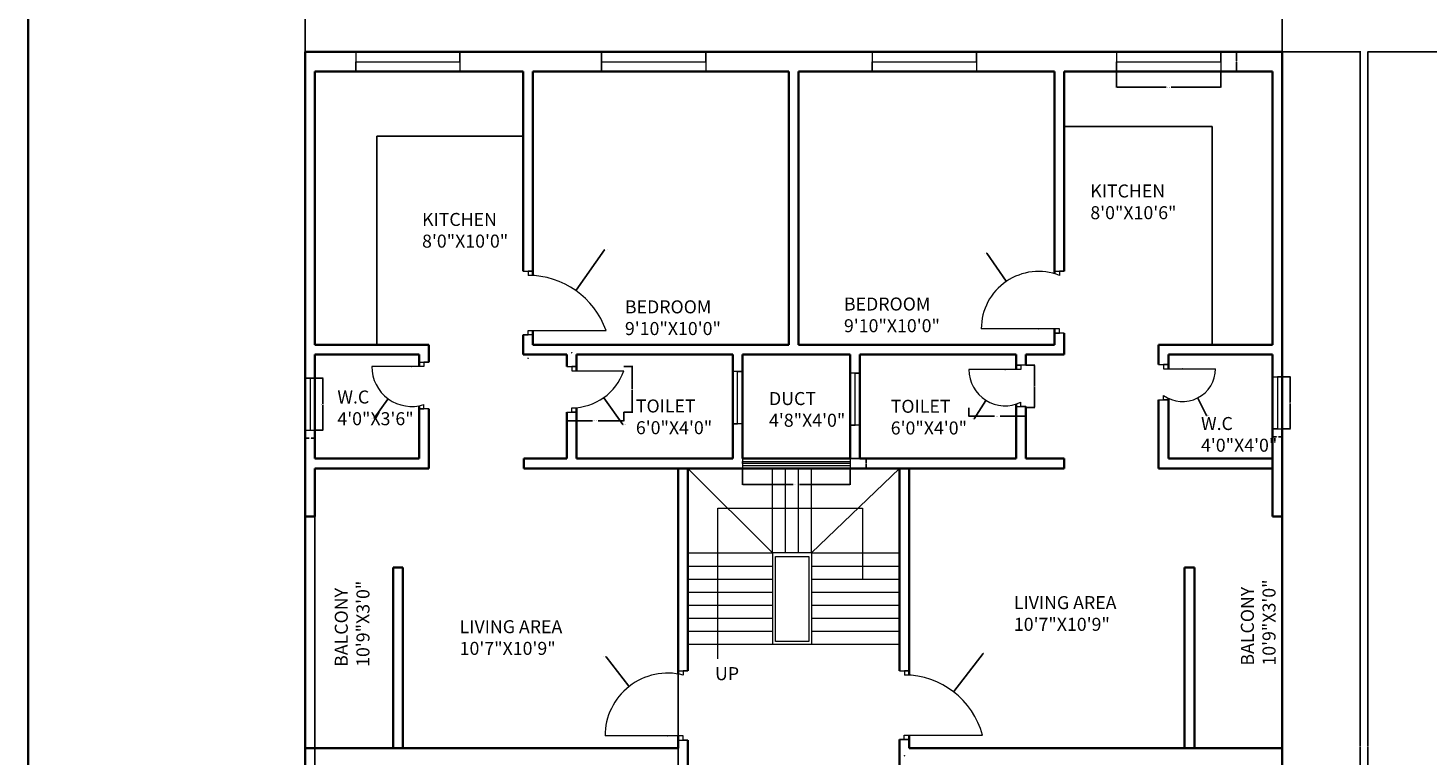
# Model space of a CAD drawing. Units: inches. Extents: x 2043 to 3387, y 1535 to 2797.
# Tile 2 of 7: x 2043 to 2688, y 2002 to 2337. Entities that reach past the tile are written whole.
import ezdxf

# ---------------------------------------------------------------- set-up
doc = ezdxf.new("R2010")
doc.units = ezdxf.units.IN
for name, color, linetype, lineweight in [('A-ANNO-DIMS', 2, 'Continuous', 18), ('A-ANNO-TEXT', 7, 'Continuous', 18), ('A-ANNO-TTLB', 7, 'Continuous', 35), ('A-AREA-IDEN', 7, 'Continuous', 18), ('A-DOOR', 3, 'Continuous', 18), ('A-FLOR-FIXT', 9, 'Continuous', 25), ('A-FLOR-STRS', 2, 'Continuous', 18), ('A-GLAZ', 4, 'Continuous', 18), ('A-WALL', 7, 'Continuous', 35)]:
    doc.layers.add(name, color=color, linetype=linetype, lineweight=lineweight)
doc.styles.get("Standard").update_dxf_attribs({"font": 'arial.ttf'})
doc.dimstyles.get("Standard").update_dxf_attribs({"dimtxt": 0.18, "dimasz": 0.18, "dimexe": 0.18, "dimexo": 0.0625, "dimgap": 0.09, "dimtad": 0, "dimtih": 1, "dimtoh": 1, "dimdec": 4, "dimzin": 0, "dimdsep": 46, "dimtxsty": 'Standard', "dimcen": 0.09, "dimadec": 0, "dimazin": 0, "dimtfac": 1, "dimtdec": 4, "dimtofl": 0, "dimtmove": 0, "dimatfit": 3, "dimfxl": 1, "dimtolj": 1, "dimtzin": 0, "dimarcsym": 0})

# ---------------------------------------------------------------- blocks, each defined once
blk = doc.blocks.new('DOOR-24-WC-NW')
for p, q in [((24, 19.53), (0, 19.53)), ((21.75, 21.53), (26.25, 21.53)), ((26.25, 21.53), (24, 21.53)), ((24, 21.53), (24, 19.53)), ((24, 0), (24, 2)), ((26.25, 0), (21.75, 0)), ((21.75, 0), (24, 0))]:
    blk.add_line(p, q)
blk.add_arc((18.4, 19.53), 18.41, 180, 287.6967)
blk = doc.blocks.new('DOOR-36-BED-NW')
for p, q in [((0, 29.41), (4.5, 29.41)), ((4.5, 29.41), (2.25, 29.41)), ((2.25, 29.41), (2.25, 27.41)), ((4.5, 0), (0, 0)), ((0, 0), (2.25, 0)), ((2.25, 0), (2.25, 2)), ((2.25, 2), (38.25, 2))]:
    blk.add_line(p, q)
blk.add_arc((2.25, -10.79), 38.2, 19.56074, 90)
blk = doc.blocks.new('DOOR-36-BED-NE')
for p, q in [((33.75, 28.58), (38.25, 28.58)), ((38.25, 28.58), (36, 28.58)), ((36, 28.58), (36, 26.58)), ((36, 2), (0, 2)), ((38.25, 0), (33.75, 0)), ((33.75, 0), (36, 0)), ((36, 0), (36, 2))]:
    blk.add_line(p, q)
blk.add_arc((26.39, 2), 26.39, 68.64806, 180)
blk = doc.blocks.new('DOOR-24-WC-NE')
for p, q in [((0, 17.14), (4.5, 17.14)), ((4.5, 17.14), (2.25, 17.14)), ((2.25, 17.14), (2.25, 15.14)), ((2.25, 15.14), (26.25, 15.14)), ((0, 0.86), (4.5, 0.86)), ((2.25, 0.86), (2.25, 2.86)), ((4.5, 0.86), (2.25, 0.86)), ((4.5, 0.86), (4.5, 0.86))]:
    blk.add_line(p, q)
blk.add_arc((11.11, 15.14), 15.14, 234.19542, 0)
blk = doc.blocks.new('DOOR-24-BATH-NW')
for p, q in [((0, 21.1), (4.5, 21.1)), ((4.5, 21.1), (2.25, 21.1)), ((2.25, 21.1), (2.25, 19.1)), ((2.25, 19.1), (26.25, 19.1)), ((2.25, 0), (2.25, 2)), ((0, 0), (4.5, 0)), ((4.5, 0), (2.25, 0))]:
    blk.add_line(p, q)
blk.add_arc((2.25, 27.39), 25.39, 270, 340.93831)
blk = doc.blocks.new('DOOR-24-BATH-NE')
for p, q in [((24, 17.07), (0, 17.07)), ((26.25, 19.07), (21.75, 19.07)), ((21.75, 19.07), (24, 19.07)), ((24, 19.07), (24, 17.07)), ((24, 0), (24, 2)), ((21.75, 0), (26.25, 0)), ((26.25, 0), (24, 0))]:
    blk.add_line(p, q)
blk.add_arc((16.73, 17.07), 16.73, 180, 295.74666)
blk = doc.blocks.new('DOOR-36-ENTRY-NW')
for p, q in [((33.75, 32.08), (38.25, 32.08)), ((38.25, 32.08), (36, 32.08)), ((36, 32.08), (36, 30.08)), ((36, 2), (0, 2)), ((33.75, 0), (38.25, 0)), ((36, 0), (36, 2)), ((38.25, 0), (36, 0))]:
    blk.add_line(p, q)
blk.add_arc((28.95, 2), 28.95, 75.89964, 180)
blk = doc.blocks.new('DOOR-36-ENTRY-NE')
for p, q in [((0, 31.7), (3.27, 31.7)), ((4.5, 31.7), (2.28, 31.7)), ((2.28, 31.7), (2.28, 29.7)), ((3.27, 31.7), (4.5, 31.7)), ((0, 0), (4.5, 0)), ((4.5, 0), (0, 0)), ((0, 0), (2.25, 0)), ((2.25, 0), (2.25, 2)), ((2.25, 2), (38.25, 2))]:
    blk.add_line(p, q)
blk.add_arc((2.28, -7.5), 37.2, 14.79344, 90)
blk = doc.blocks.new('COUNTER-L-NW')
for p, q in [((67.52, 96.23), (0, 96.23)), ((0, 96.23), (0, 0))]:
    blk.add_line(p, q)
blk = doc.blocks.new('COUNTER-L-NE')
for p, q in [((0, 100.61), (68.19, 100.61)), ((68.19, 100.61), (68.19, 0))]:
    blk.add_line(p, q)
blk = doc.blocks.new('STAIR-U-RETURN')
for p, q in [((0, 87.81), (0, 48.81)), ((39, 48.81), (0, 87.81)), ((39, 48.81), (39, 87.81)), ((45, 48.81), (45, 87.81)), ((51, 48.81), (51, 87.81)), ((57, 48.81), (57, 87.81)), ((57, 48.81), (97.5, 87.81)), ((97.5, 87.81), (58.5, 87.81)), ((13.82, 0), (13.82, 69.54)), ((13.82, 69.54), (80.42, 69.54)), ((80.42, 69.54), (80.42, 36.81)), ((0, 48.81), (39, 48.81)), ((57, 48.81), (39, 48.81)), ((39, 48.81), (39, 48.81)), ((39, 48.81), (39, 6.81)), ((57, 48.81), (57, 6.81)), ((57, 48.81), (97.5, 48.81)), ((0, 42.81), (39, 42.81)), ((57, 42.81), (97.5, 42.81)), ((0, 36.81), (39, 36.81)), ((57, 36.81), (97.5, 36.81)), ((0, 30.81), (39, 30.81)), ((57, 30.81), (97.5, 30.81)), ((0, 24.81), (39, 24.81)), ((57, 24.81), (97.5, 24.81)), ((0, 18.81), (39, 18.81)), ((57, 18.81), (97.5, 18.81)), ((0, 12.81), (39, 12.81)), ((0, 6.81), (39, 6.81)), ((39, 6.81), (57, 6.81)), ((57, 12.81), (97.5, 12.81)), ((57, 6.81), (97.5, 6.81))]:
    blk.add_line(p, q)
blk.add_lwpolyline([(40.29, 47.17), (55.75, 47.17), (55.75, 8.03), (40.29, 8.03)], close=True)
blk = doc.blocks.new('WIN-48-PLAN')
for p, q in [((0, 9), (0, 0)), ((48, 4.5), (48, 9)), ((48, 9), (48, 0)), ((0, 0), (0, 4.5)), ((0, 4.5), (48, 4.5))]:
    blk.add_line(p, q)
blk = doc.blocks.new('WIN-48-N-JAMB')
for p, q in [((0, 9), (0, 0)), ((0, 0), (0, 9)), ((0, 9), (0, 4.5)), ((48, 4.5), (48, 9)), ((48, 9), (48, 0)), ((0, 4.5), (48, 4.5))]:
    blk.add_line(p, q)
blk = doc.blocks.new('VENT-24-W')
for p, q in [((0, 24), (4.5, 24)), ((4.5, 24), (0, 24)), ((0, 24), (0, 0)), ((2.25, 24), (2.25, 0)), ((0, 0), (4.5, 0))]:
    blk.add_line(p, q)
blk = doc.blocks.new('VENT-24-PLAN')
for p, q in [((0, 24), (4.5, 24)), ((4.5, 24), (2.25, 24)), ((2.25, 24), (2.25, 0)), ((2.25, 0), (0, 0)), ((0, 0), (4.5, 0))]:
    blk.add_line(p, q)
blk = doc.blocks.new('WIN-STAIR-DUCT')
for p, q in [((0, 4.5), (0, 0)), ((0, 2.25), (0, 3.25)), ((0, 3.25), (49.62, 3.25)), ((49.62, 2.25), (0, 2.25)), ((49.62, 1.25), (0, 1.25)), ((49.62, 4.5), (49.62, 0)), ((49.62, 3.25), (49.62, 2.25)), ((49.62, 2.25), (49.62, 2.25)), ((49.62, 2.25), (49.62, 1.25))]:
    blk.add_line(p, q)
blk = doc.blocks.new('*D35')
at = {"layer": 'A-ANNO-DIMS', "color": 0, "lineweight": -2, "transparency": 16777216}
for p, q in [((2620.91, 2176.55), (2624.63, 2176.55)), ((2624.45, 2176.37), (2624.45, 2164.73)), ((2624.45, 2152.73), (2624.45, 2164.37)), ((2620.91, 2152.55), (2624.63, 2152.55))]:
    blk.add_line(p, q, dxfattribs=at)
at = {"layer": 'A-ANNO-DIMS', "color": 0, "transparency": 16777216}
for points in [[(2624.42, 2176.37), (2624.48, 2176.37), (2624.45, 2176.55)], [(2624.42, 2152.73), (2624.48, 2152.73), (2624.45, 2152.55)]]:
    blk.add_solid(points, dxfattribs=at)
at = {"layer": 'Defpoints', "color": 0, "transparency": 16777216}
for p in [(2620.85, 2176.55), (2624.45, 2176.55), (2620.85, 2152.55)]:
    blk.add_point(p, dxfattribs=at)
at = {"layer": 'A-ANNO-DIMS', "color": 0, "transparency": 16777216, "insert": (2624.45, 2164.55), "char_height": 0.18, "attachment_point": 5}
blk.add_mtext('\\A1;VENT 24 TYP.', dxfattribs=at)
blk = doc.blocks.new('*D36')
at = {"layer": 'A-ANNO-DIMS', "color": 0, "lineweight": -2, "transparency": 16777216}
for p, q in [((2616.35, 2152.48), (2616.35, 2148.77)), ((2620.85, 2152.48), (2620.85, 2148.77)), ((2616.53, 2148.95), (2618.14, 2148.95)), ((2620.67, 2148.95), (2619.06, 2148.95))]:
    blk.add_line(p, q, dxfattribs=at)
at = {"layer": 'A-ANNO-DIMS', "color": 0, "transparency": 16777216}
for points in [[(2616.53, 2148.98), (2616.53, 2148.92), (2616.35, 2148.95)], [(2620.67, 2148.98), (2620.67, 2148.92), (2620.85, 2148.95)]]:
    blk.add_solid(points, dxfattribs=at)
at = {"layer": 'Defpoints', "color": 0, "transparency": 16777216}
for p in [(2616.35, 2152.55), (2620.85, 2152.55), (2620.85, 2148.95)]:
    blk.add_point(p, dxfattribs=at)
at = {"layer": 'A-ANNO-DIMS', "color": 0, "transparency": 16777216, "insert": (2618.6, 2148.95), "char_height": 0.18, "attachment_point": 5}
blk.add_mtext('\\A1;5 TYP.', dxfattribs=at)
blk = doc.blocks.new('*D37')
at = {"layer": 'A-ANNO-DIMS', "color": 0, "lineweight": -2, "transparency": 16777216}
for p, q in [((2544.5, 2317.31), (2544.5, 2310)), ((2592.5, 2317.31), (2592.5, 2310)), ((2544.68, 2310.18), (2567.38, 2310.18)), ((2592.32, 2310.18), (2569.62, 2310.18))]:
    blk.add_line(p, q, dxfattribs=at)
at = {"layer": 'A-ANNO-DIMS', "color": 0, "transparency": 16777216}
for points in [[(2544.68, 2310.21), (2544.68, 2310.15), (2544.5, 2310.18)], [(2592.32, 2310.21), (2592.32, 2310.15), (2592.5, 2310.18)]]:
    blk.add_solid(points, dxfattribs=at)
at = {"layer": 'Defpoints', "color": 0, "transparency": 16777216}
for p in [(2544.5, 2317.38), (2592.5, 2317.38), (2592.5, 2310.18)]:
    blk.add_point(p, dxfattribs=at)
at = {"layer": 'A-ANNO-DIMS', "color": 0, "transparency": 16777216, "insert": (2568.5, 2310.18), "char_height": 0.18, "attachment_point": 5}
blk.add_mtext('\\A1;WINDOW 48 TYP.', dxfattribs=at)
blk = doc.blocks.new('*D38')
at = {"layer": 'A-ANNO-DIMS', "color": 0, "lineweight": -2, "transparency": 16777216}
for p, q in [((2592.57, 2326.38), (2599.88, 2326.38)), ((2599.7, 2326.2), (2599.7, 2322.06)), ((2599.7, 2317.56), (2599.7, 2321.7)), ((2592.57, 2317.38), (2599.88, 2317.38))]:
    blk.add_line(p, q, dxfattribs=at)
at = {"layer": 'A-ANNO-DIMS', "color": 0, "transparency": 16777216}
for points in [[(2599.67, 2326.2), (2599.73, 2326.2), (2599.7, 2326.38)], [(2599.67, 2317.56), (2599.73, 2317.56), (2599.7, 2317.38)]]:
    blk.add_solid(points, dxfattribs=at)
at = {"layer": 'Defpoints', "color": 0, "transparency": 16777216}
for p in [(2592.5, 2326.38), (2599.7, 2326.38), (2592.5, 2317.38)]:
    blk.add_point(p, dxfattribs=at)
at = {"layer": 'A-ANNO-DIMS', "color": 0, "transparency": 16777216, "insert": (2599.7, 2321.88), "char_height": 0.18, "attachment_point": 5}
blk.add_mtext('\\A1;9 TYP.', dxfattribs=at)
blk = doc.blocks.new('*D43')
at = {"layer": 'A-ANNO-DIMS', "color": 0, "lineweight": -2, "transparency": 16777216}
for p, q in [((2174.91, 2175.93), (2178.63, 2175.93)), ((2178.45, 2175.75), (2178.45, 2164.11)), ((2178.45, 2152.11), (2178.45, 2163.75)), ((2174.91, 2151.93), (2178.63, 2151.93))]:
    blk.add_line(p, q, dxfattribs=at)
at = {"layer": 'A-ANNO-DIMS', "color": 0, "transparency": 16777216}
for points in [[(2178.42, 2175.75), (2178.48, 2175.75), (2178.45, 2175.93)], [(2178.42, 2152.11), (2178.48, 2152.11), (2178.45, 2151.93)]]:
    blk.add_solid(points, dxfattribs=at)
at = {"layer": 'Defpoints', "color": 0, "transparency": 16777216}
for p in [(2174.85, 2175.93), (2178.45, 2175.93), (2174.85, 2151.93)]:
    blk.add_point(p, dxfattribs=at)
at = {"layer": 'A-ANNO-DIMS', "color": 0, "transparency": 16777216, "insert": (2178.45, 2163.93), "char_height": 0.18, "attachment_point": 5}
blk.add_mtext('\\A1;VENT 24 TYP.', dxfattribs=at)
blk = doc.blocks.new('*D44')
at = {"layer": 'A-ANNO-DIMS', "color": 0, "lineweight": -2, "transparency": 16777216}
for p, q in [((2170.35, 2151.87), (2170.35, 2148.15)), ((2174.85, 2151.87), (2174.85, 2148.15)), ((2170.53, 2148.33), (2172.14, 2148.33)), ((2174.67, 2148.33), (2173.06, 2148.33))]:
    blk.add_line(p, q, dxfattribs=at)
at = {"layer": 'A-ANNO-DIMS', "color": 0, "transparency": 16777216}
for points in [[(2170.53, 2148.36), (2170.53, 2148.3), (2170.35, 2148.33)], [(2174.67, 2148.36), (2174.67, 2148.3), (2174.85, 2148.33)]]:
    blk.add_solid(points, dxfattribs=at)
at = {"layer": 'Defpoints', "color": 0, "transparency": 16777216}
for p in [(2170.35, 2151.93), (2174.85, 2151.93), (2174.85, 2148.33)]:
    blk.add_point(p, dxfattribs=at)
at = {"layer": 'A-ANNO-DIMS', "color": 0, "transparency": 16777216, "insert": (2172.6, 2148.33), "char_height": 0.18, "attachment_point": 5}
blk.add_mtext('\\A1;5 TYP.', dxfattribs=at)
blk = doc.blocks.new('*D45')
at = {"layer": 'A-ANNO-DIMS', "color": 0, "lineweight": -2, "transparency": 16777216}
for p, q in [((2372.01, 2134.31), (2372.01, 2126.75)), ((2421.63, 2134.31), (2421.63, 2126.75)), ((2372.19, 2126.93), (2395.32, 2126.93)), ((2421.45, 2126.93), (2398.31, 2126.93))]:
    blk.add_line(p, q, dxfattribs=at)
at = {"layer": 'A-ANNO-DIMS', "color": 0, "transparency": 16777216}
for points in [[(2372.19, 2126.96), (2372.19, 2126.9), (2372.01, 2126.93)], [(2421.45, 2126.96), (2421.45, 2126.9), (2421.63, 2126.93)]]:
    blk.add_solid(points, dxfattribs=at)
at = {"layer": 'Defpoints', "color": 0, "transparency": 16777216}
for p in [(2372.01, 2134.38), (2421.63, 2134.38), (2421.63, 2126.93)]:
    blk.add_point(p, dxfattribs=at)
at = {"layer": 'A-ANNO-DIMS', "color": 0, "transparency": 16777216, "insert": (2396.82, 2126.93), "char_height": 0.18, "attachment_point": 5}
blk.add_mtext('\\A1;DUCT WINDOW 50 TYP.', dxfattribs=at)
blk = doc.blocks.new('*D46')
at = {"layer": 'A-ANNO-DIMS', "color": 0, "lineweight": -2, "transparency": 16777216}
for p, q in [((2421.69, 2138.88), (2429.25, 2138.88)), ((2429.07, 2138.7), (2429.07, 2136.81)), ((2421.69, 2134.38), (2429.25, 2134.38)), ((2429.07, 2134.56), (2429.07, 2136.45))]:
    blk.add_line(p, q, dxfattribs=at)
at = {"layer": 'A-ANNO-DIMS', "color": 0, "transparency": 16777216}
for points in [[(2429.04, 2138.7), (2429.1, 2138.7), (2429.07, 2138.88)], [(2429.04, 2134.56), (2429.1, 2134.56), (2429.07, 2134.38)]]:
    blk.add_solid(points, dxfattribs=at)
at = {"layer": 'Defpoints', "color": 0, "transparency": 16777216}
for p in [(2421.63, 2138.88), (2429.07, 2138.88), (2421.63, 2134.38)]:
    blk.add_point(p, dxfattribs=at)
at = {"layer": 'A-ANNO-DIMS', "color": 0, "transparency": 16777216, "insert": (2429.07, 2136.63), "char_height": 0.18, "attachment_point": 5}
blk.add_mtext('\\A1;5 TYP.', dxfattribs=at)
blk = doc.blocks.new('*D57')
at = {"layer": 'A-ANNO-DIMS', "color": 0, "lineweight": -2, "transparency": 16777216}
for p, q in [((2291.01, 2160.23), (2291.01, 2156.18)), ((2291.19, 2156.36), (2302.82, 2156.36)), ((2317.08, 2156.36), (2305.44, 2156.36)), ((2317.26, 2160.23), (2317.26, 2156.18))]:
    blk.add_line(p, q, dxfattribs=at)
at = {"layer": 'A-ANNO-DIMS', "color": 0, "transparency": 16777216}
for points in [[(2291.19, 2156.39), (2291.19, 2156.33), (2291.01, 2156.36)], [(2317.08, 2156.39), (2317.08, 2156.33), (2317.26, 2156.36)]]:
    blk.add_solid(points, dxfattribs=at)
at = {"layer": 'Defpoints', "color": 0, "transparency": 16777216}
for p in [(2291.01, 2160.29), (2317.26, 2160.29), (2317.26, 2156.36)]:
    blk.add_point(p, dxfattribs=at)
at = {"layer": 'A-ANNO-DIMS', "color": 0, "transparency": 16777216, "insert": (2304.13, 2156.36), "char_height": 0.18, "attachment_point": 5}
blk.add_mtext('\\A1;BATH DOOR 26 TYP.', dxfattribs=at)
blk = doc.blocks.new('*D58')
at = {"layer": 'A-ANNO-DIMS', "color": 0, "lineweight": -2, "transparency": 16777216}
for p, q in [((2317.32, 2181.39), (2321.37, 2181.39)), ((2321.19, 2181.21), (2321.19, 2171.02)), ((2321.19, 2160.47), (2321.19, 2170.66)), ((2317.32, 2160.29), (2321.37, 2160.29))]:
    blk.add_line(p, q, dxfattribs=at)
at = {"layer": 'A-ANNO-DIMS', "color": 0, "transparency": 16777216}
for points in [[(2321.16, 2181.21), (2321.22, 2181.21), (2321.19, 2181.39)], [(2321.16, 2160.47), (2321.22, 2160.47), (2321.19, 2160.29)]]:
    blk.add_solid(points, dxfattribs=at)
at = {"layer": 'Defpoints', "color": 0, "transparency": 16777216}
for p in [(2317.26, 2181.39), (2321.19, 2181.39), (2317.26, 2160.29)]:
    blk.add_point(p, dxfattribs=at)
at = {"layer": 'A-ANNO-DIMS', "color": 0, "transparency": 16777216, "insert": (2321.19, 2170.84), "char_height": 0.18, "attachment_point": 5}
blk.add_mtext('\\A1;21 TYP.', dxfattribs=at)
blk = doc.blocks.new('*D59')
at = {"layer": 'A-ANNO-DIMS', "color": 0, "lineweight": -2, "transparency": 16777216}
for p, q in [((2476.38, 2162.31), (2476.38, 2158.26)), ((2476.56, 2158.44), (2488.2, 2158.44)), ((2502.45, 2158.44), (2490.81, 2158.44)), ((2502.63, 2162.31), (2502.63, 2158.26))]:
    blk.add_line(p, q, dxfattribs=at)
at = {"layer": 'A-ANNO-DIMS', "color": 0, "transparency": 16777216}
for points in [[(2476.56, 2158.47), (2476.56, 2158.41), (2476.38, 2158.44)], [(2502.45, 2158.47), (2502.45, 2158.41), (2502.63, 2158.44)]]:
    blk.add_solid(points, dxfattribs=at)
at = {"layer": 'Defpoints', "color": 0, "transparency": 16777216}
for p in [(2476.38, 2162.38), (2502.63, 2162.38), (2502.63, 2158.44)]:
    blk.add_point(p, dxfattribs=at)
at = {"layer": 'A-ANNO-DIMS', "color": 0, "transparency": 16777216, "insert": (2489.5, 2158.44), "char_height": 0.18, "attachment_point": 5}
blk.add_mtext('\\A1;BATH DOOR 26 TYP.', dxfattribs=at)
blk = doc.blocks.new('*D60')
at = {"layer": 'A-ANNO-DIMS', "color": 0, "lineweight": -2, "transparency": 16777216}
for p, q in [((2502.69, 2181.95), (2506.75, 2181.95)), ((2506.57, 2181.77), (2506.57, 2172.34)), ((2506.57, 2162.56), (2506.57, 2171.98)), ((2502.69, 2162.38), (2506.75, 2162.38))]:
    blk.add_line(p, q, dxfattribs=at)
at = {"layer": 'A-ANNO-DIMS', "color": 0, "transparency": 16777216}
for points in [[(2506.54, 2181.77), (2506.6, 2181.77), (2506.57, 2181.95)], [(2506.54, 2162.56), (2506.6, 2162.56), (2506.57, 2162.38)]]:
    blk.add_solid(points, dxfattribs=at)
at = {"layer": 'Defpoints', "color": 0, "transparency": 16777216}
for p in [(2502.63, 2181.95), (2506.57, 2181.95), (2502.63, 2162.38)]:
    blk.add_point(p, dxfattribs=at)
at = {"layer": 'A-ANNO-DIMS', "color": 0, "transparency": 16777216, "insert": (2506.57, 2172.16), "char_height": 0.18, "attachment_point": 5}
blk.add_mtext('\\A1;20 TYP.', dxfattribs=at)
blk = doc.blocks.new('*D103')
at = {"layer": 'A-ANNO-DIMS', "color": 0, "lineweight": -2, "transparency": 16777216}
for p, q in [((2170.35, 2326.44), (2170.35, 2362.56)), ((2170.53, 2362.38), (2395.2, 2362.38)), ((2620.67, 2362.38), (2396, 2362.38)), ((2620.85, 2326.44), (2620.85, 2362.56))]:
    blk.add_line(p, q, dxfattribs=at)
at = {"layer": 'A-ANNO-DIMS', "color": 0, "transparency": 16777216}
for points in [[(2170.53, 2362.41), (2170.53, 2362.35), (2170.35, 2362.38)], [(2620.67, 2362.41), (2620.67, 2362.35), (2620.85, 2362.38)]]:
    blk.add_solid(points, dxfattribs=at)
at = {"layer": 'Defpoints', "color": 0, "transparency": 16777216}
for p in [(2620.85, 2362.38), (2170.35, 2326.38), (2620.85, 2326.38)]:
    blk.add_point(p, dxfattribs=at)
at = {"layer": 'A-ANNO-DIMS', "color": 0, "transparency": 16777216, "insert": (2395.6, 2362.38), "char_height": 0.18, "attachment_point": 5}
blk.add_mtext('\\A1;450.5', dxfattribs=at)
blk = doc.blocks.new('*D104')
at = {"layer": 'A-ANNO-DIMS', "color": 0, "lineweight": -2, "transparency": 16777216}
for p, q in [((2620.91, 2326.38), (2657.03, 2326.38)), ((2656.85, 2326.2), (2656.85, 2006.31)), ((2656.85, 1686.06), (2656.85, 2005.95)), ((2620.91, 1685.88), (2657.03, 1685.88))]:
    blk.add_line(p, q, dxfattribs=at)
at = {"layer": 'A-ANNO-DIMS', "color": 0, "transparency": 16777216}
for points in [[(2656.82, 2326.2), (2656.88, 2326.2), (2656.85, 2326.38)], [(2656.82, 1686.06), (2656.88, 1686.06), (2656.85, 1685.88)]]:
    blk.add_solid(points, dxfattribs=at)
at = {"layer": 'Defpoints', "color": 0, "transparency": 16777216}
for p in [(2620.85, 2326.38), (2656.85, 2326.38), (2620.85, 1685.88)]:
    blk.add_point(p, dxfattribs=at)
at = {"layer": 'A-ANNO-DIMS', "color": 0, "transparency": 16777216, "insert": (2656.85, 2006.13), "char_height": 0.18, "attachment_point": 5}
blk.add_mtext('\\A1;640.5', dxfattribs=at)
blk = doc.blocks.new('*D106')
at = {"layer": 'A-ANNO-DIMS', "color": 0, "lineweight": -2, "transparency": 16777216}
for p, q in [((2723.65, 2326.38), (2660.13, 2326.38)), ((2660.31, 2326.2), (2660.31, 2006.31)), ((2660.31, 1686.06), (2660.31, 2005.95)), ((2723.65, 1685.88), (2660.13, 1685.88))]:
    blk.add_line(p, q, dxfattribs=at)
at = {"layer": 'A-ANNO-DIMS', "color": 0, "transparency": 16777216}
for points in [[(2660.28, 2326.2), (2660.34, 2326.2), (2660.31, 2326.38)], [(2660.28, 1686.06), (2660.34, 1686.06), (2660.31, 1685.88)]]:
    blk.add_solid(points, dxfattribs=at)
at = {"layer": 'Defpoints', "color": 0, "transparency": 16777216}
for p in [(2660.31, 2326.38), (2723.71, 2326.38), (2723.71, 1685.88)]:
    blk.add_point(p, dxfattribs=at)
at = {"layer": 'A-ANNO-DIMS', "color": 0, "transparency": 16777216, "insert": (2660.31, 2006.13), "char_height": 0.18, "attachment_point": 5}
blk.add_mtext('\\A1;640.5', dxfattribs=at)
blk = doc.blocks.new('*D117')
at = {"layer": 'A-ANNO-DIMS', "color": 0, "lineweight": -2, "transparency": 16777216}
for p, q in [((2174.85, 2134.31), (2174.85, 1649.7)), ((2342.35, 2134.31), (2342.35, 1649.7)), ((2175.03, 1649.88), (2258.21, 1649.88)), ((2342.17, 1649.88), (2258.99, 1649.88))]:
    blk.add_line(p, q, dxfattribs=at)
at = {"layer": 'A-ANNO-DIMS', "color": 0, "transparency": 16777216}
for points in [[(2175.03, 1649.91), (2175.03, 1649.85), (2174.85, 1649.88)], [(2342.17, 1649.91), (2342.17, 1649.85), (2342.35, 1649.88)]]:
    blk.add_solid(points, dxfattribs=at)
at = {"layer": 'Defpoints', "color": 0, "transparency": 16777216}
for p in [(2174.85, 2134.38), (2342.35, 2134.38), (2342.35, 1649.88)]:
    blk.add_point(p, dxfattribs=at)
at = {"layer": 'A-ANNO-DIMS', "color": 0, "transparency": 16777216, "insert": (2258.6, 1649.88), "char_height": 0.18, "attachment_point": 5}
blk.add_mtext('\\A1;167.5', dxfattribs=at)
blk = doc.blocks.new('*D133')
at = {"layer": 'A-ANNO-DIMS', "color": 0, "lineweight": -2, "transparency": 16777216}
for p, q in [((2308.35, 2235.09), (2295.24, 2216.51)), ((2308.53, 2235.09), (2308.35, 2235.09)), ((2273.01, 2185.15), (2273.19, 2185.15)), ((2273.1, 2185.06), (2273.1, 2185.24))]:
    blk.add_line(p, q, dxfattribs=at)
at = {"layer": 'A-ANNO-DIMS', "color": 0, "transparency": 16777216}
blk.add_solid([(2295.21, 2216.53), (2295.26, 2216.49), (2295.13, 2216.36)], dxfattribs=at)
at = {"layer": 'Defpoints', "color": 0, "transparency": 16777216}
for p in [(2295.13, 2216.36), (2273.1, 2185.15)]:
    blk.add_point(p, dxfattribs=at)
at = {"layer": 'A-ANNO-DIMS', "color": 0, "transparency": 16777216, "insert": (2309.28, 2235.09), "char_height": 0.18, "attachment_point": 5}
blk.add_mtext('\\A1;2X R38.205', dxfattribs=at)
blk = doc.blocks.new('*D135')
at = {"layer": 'A-ANNO-DIMS', "color": 0, "lineweight": -2, "transparency": 16777216}
for p, q in [((2482.95, 2049.08), (2469.44, 2031.54)), ((2483.13, 2049.08), (2482.95, 2049.08)), ((2446.54, 2001.92), (2446.72, 2001.92)), ((2446.63, 2001.83), (2446.63, 2002.01))]:
    blk.add_line(p, q, dxfattribs=at)
at = {"layer": 'A-ANNO-DIMS', "color": 0, "transparency": 16777216}
blk.add_solid([(2469.42, 2031.55), (2469.47, 2031.52), (2469.33, 2031.39)], dxfattribs=at)
at = {"layer": 'Defpoints', "color": 0, "transparency": 16777216}
for p in [(2469.33, 2031.39), (2446.63, 2001.92)]:
    blk.add_point(p, dxfattribs=at)
at = {"layer": 'A-ANNO-DIMS', "color": 0, "transparency": 16777216, "insert": (2483.74, 2049.08), "char_height": 0.18, "attachment_point": 5}
blk.add_mtext('\\A1;2X R37.2', dxfattribs=at)
blk = doc.blocks.new('*D137')
at = {"layer": 'A-ANNO-DIMS', "color": 0, "lineweight": -2, "transparency": 16777216}
for p, q in [((2308.88, 2047.57), (2309.06, 2047.57)), ((2309.06, 2047.57), (2319.63, 2034.01)), ((2337.46, 2011.05), (2337.64, 2011.05)), ((2337.55, 2010.96), (2337.55, 2011.14))]:
    blk.add_line(p, q, dxfattribs=at)
at = {"layer": 'A-ANNO-DIMS', "color": 0, "transparency": 16777216}
blk.add_solid([(2319.66, 2034.03), (2319.61, 2034), (2319.75, 2033.87)], dxfattribs=at)
at = {"layer": 'Defpoints', "color": 0, "transparency": 16777216}
for p in [(2319.75, 2033.87), (2337.55, 2011.05)]:
    blk.add_point(p, dxfattribs=at)
at = {"layer": 'A-ANNO-DIMS', "color": 0, "transparency": 16777216, "insert": (2308.21, 2047.57), "char_height": 0.18, "attachment_point": 5}
blk.add_mtext('\\A1;2X R28.95', dxfattribs=at)
blk = doc.blocks.new('*D140')
at = {"layer": 'A-ANNO-DIMS', "color": 0, "lineweight": -2, "transparency": 16777216}
for p, q in [((2484.5, 2233.65), (2484.68, 2233.65)), ((2484.68, 2233.65), (2493.51, 2220.72)), ((2508.4, 2198.78), (2508.58, 2198.78)), ((2508.49, 2198.69), (2508.49, 2198.87))]:
    blk.add_line(p, q, dxfattribs=at)
at = {"layer": 'A-ANNO-DIMS', "color": 0, "transparency": 16777216}
blk.add_solid([(2493.53, 2220.74), (2493.48, 2220.7), (2493.61, 2220.57)], dxfattribs=at)
at = {"layer": 'Defpoints', "color": 0, "transparency": 16777216}
for p in [(2493.61, 2220.57), (2508.49, 2198.78)]:
    blk.add_point(p, dxfattribs=at)
at = {"layer": 'A-ANNO-DIMS', "color": 0, "transparency": 16777216, "insert": (2483.83, 2233.65), "char_height": 0.18, "attachment_point": 5}
blk.add_mtext('\\A1;2X R26.39', dxfattribs=at)
blk = doc.blocks.new('*D141')
at = {"layer": 'A-ANNO-DIMS', "color": 0, "lineweight": -2, "transparency": 16777216}
for p, q in [((2293.17, 2187.69), (2293.35, 2187.69)), ((2293.26, 2187.6), (2293.26, 2187.78)), ((2316.83, 2154.6), (2308.09, 2166.86)), ((2317.01, 2154.6), (2316.83, 2154.6))]:
    blk.add_line(p, q, dxfattribs=at)
at = {"layer": 'A-ANNO-DIMS', "color": 0, "transparency": 16777216}
blk.add_solid([(2308.12, 2166.88), (2308.07, 2166.84), (2307.99, 2167.01)], dxfattribs=at)
at = {"layer": 'Defpoints', "color": 0, "transparency": 16777216}
for p in [(2293.26, 2187.69), (2307.99, 2167.01)]:
    blk.add_point(p, dxfattribs=at)
at = {"layer": 'A-ANNO-DIMS', "color": 0, "transparency": 16777216, "insert": (2317.68, 2154.6), "char_height": 0.18, "attachment_point": 5}
blk.add_mtext('\\A1;2X R25.39', dxfattribs=at)
blk = doc.blocks.new('*D145')
at = {"layer": 'A-ANNO-DIMS', "color": 0, "lineweight": -2, "transparency": 16777216}
for p, q in [((2219.41, 2181.33), (2219.59, 2181.33)), ((2219.5, 2181.24), (2219.5, 2181.42)), ((2202.13, 2157.55), (2208.54, 2166.32)), ((2201.95, 2157.55), (2202.13, 2157.55))]:
    blk.add_line(p, q, dxfattribs=at)
at = {"layer": 'A-ANNO-DIMS', "color": 0, "transparency": 16777216}
blk.add_solid([(2208.52, 2166.34), (2208.56, 2166.3), (2208.65, 2166.47)], dxfattribs=at)
at = {"layer": 'Defpoints', "color": 0, "transparency": 16777216}
for p in [(2219.5, 2181.33), (2208.65, 2166.47)]:
    blk.add_point(p, dxfattribs=at)
at = {"layer": 'A-ANNO-DIMS', "color": 0, "transparency": 16777216, "insert": (2201.21, 2157.55), "char_height": 0.18, "attachment_point": 5}
blk.add_mtext('\\A1;2X R18.405', dxfattribs=at)
blk = doc.blocks.new('*D147')
at = {"layer": 'A-ANNO-DIMS', "color": 0, "lineweight": -2, "transparency": 16777216}
for p, q in [((2493.02, 2179.95), (2493.2, 2179.95)), ((2493.11, 2179.86), (2493.11, 2180.04)), ((2478.87, 2157.28), (2484.12, 2165.63)), ((2478.69, 2157.28), (2478.87, 2157.28))]:
    blk.add_line(p, q, dxfattribs=at)
at = {"layer": 'A-ANNO-DIMS', "color": 0, "transparency": 16777216}
blk.add_solid([(2484.09, 2165.64), (2484.14, 2165.61), (2484.21, 2165.78)], dxfattribs=at)
at = {"layer": 'Defpoints', "color": 0, "transparency": 16777216}
for p in [(2493.11, 2179.95), (2484.21, 2165.78)]:
    blk.add_point(p, dxfattribs=at)
at = {"layer": 'A-ANNO-DIMS', "color": 0, "transparency": 16777216, "insert": (2477.95, 2157.28), "char_height": 0.18, "attachment_point": 5}
blk.add_mtext('\\A1;2X R16.732', dxfattribs=at)
blk = doc.blocks.new('*D148')
at = {"layer": 'A-ANNO-DIMS', "color": 0, "lineweight": -2, "transparency": 16777216}
for p, q in [((2574.87, 2180.33), (2575.05, 2180.33)), ((2574.96, 2180.24), (2574.96, 2180.42)), ((2585.99, 2158.77), (2581.94, 2166.69)), ((2586.17, 2158.77), (2585.99, 2158.77))]:
    blk.add_line(p, q, dxfattribs=at)
at = {"layer": 'A-ANNO-DIMS', "color": 0, "transparency": 16777216}
blk.add_solid([(2581.96, 2166.71), (2581.91, 2166.68), (2581.85, 2166.85)], dxfattribs=at)
at = {"layer": 'Defpoints', "color": 0, "transparency": 16777216}
for p in [(2574.96, 2180.33), (2581.85, 2166.85)]:
    blk.add_point(p, dxfattribs=at)
at = {"layer": 'A-ANNO-DIMS', "color": 0, "transparency": 16777216, "insert": (2586.92, 2158.77), "char_height": 0.18, "attachment_point": 5}
blk.add_mtext('\\A1;2X R15.142', dxfattribs=at)

msp = doc.modelspace()

# ---------------------------------------------------------------- linework, layer by layer
at = {"layer": 'A-ANNO-TTLB'}
msp.add_lwpolyline([(2042.5541, 2796.7818), (3386.9704, 2796.7818), (3386.9704, 1534.5689), (2042.5541, 1534.5689)], close=True, dxfattribs=at)
at = {"layer": 'A-WALL'}
for p, q in [((2170.3496, 2326.3769), (2620.8496, 2326.3769)), ((2174.8496, 2326.3769), (2170.3496, 2326.3769)), ((2170.3496, 2326.3769), (2170.3496, 1734.4589)), ((2620.8496, 2326.3769), (2620.8496, 1685.8769)), ((2174.8496, 2317.3769), (2270.8496, 2317.3769)), ((2174.8496, 2317.3769), (2174.8496, 2191.3769)), ((2270.8496, 2317.3769), (2270.8496, 2225.357)), ((2275.3496, 2317.3769), (2275.3496, 2223.2907)), ((2275.3496, 2317.3769), (2393.3496, 2317.3769)), ((2393.3496, 2317.3769), (2393.3496, 2191.3769)), ((2397.8496, 2317.3769), (2397.8496, 2191.3769)), ((2397.8496, 2317.3769), (2515.8496, 2317.3769)), ((2515.8496, 2317.3769), (2515.8496, 2224.1217)), ((2520.3496, 2317.3769), (2520.3496, 2225.357)), ((2520.3496, 2317.3769), (2616.3496, 2317.3769)), ((2616.3496, 2317.3769), (2616.3496, 2191.3769)), ((2270.8496, 2195.9433), (2270.8496, 2186.8769)), ((2275.3496, 2197.9433), (2275.3496, 2191.3769)), ((2515.8496, 2198.7773), (2515.8496, 2191.3769)), ((2520.3496, 2196.7773), (2520.3496, 2186.8769)), ((2174.8496, 2191.3769), (2227.3496, 2191.3769)), ((2227.3496, 2183.3291), (2227.3496, 2191.3769)), ((2275.3496, 2191.3769), (2393.3496, 2191.3769)), ((2397.8496, 2191.3769), (2515.8496, 2191.3769)), ((2563.8496, 2191.3769), (2616.3496, 2191.3769)), ((2563.8496, 2182.3328), (2563.8496, 2191.3769)), ((2174.8496, 2186.8769), (2222.8496, 2186.8769)), ((2174.8496, 2186.8769), (2174.8496, 2138.8769)), ((2174.8496, 2186.8769), (2222.8496, 2186.8769)), ((2222.8496, 2186.8769), (2222.8496, 2181.3291)), ((2270.8496, 2186.8769), (2291.0051, 2186.8769)), ((2270.8496, 2186.8769), (2291.0051, 2186.8769)), ((2291.0051, 2181.3932), (2291.0051, 2186.8769)), ((2367.5051, 2186.8769), (2295.5051, 2186.8769)), ((2295.5051, 2179.3932), (2295.5051, 2186.8769)), ((2295.5051, 2186.8769), (2342.8496, 2186.8769)), ((2295.5051, 2186.8769), (2367.5051, 2186.8769)), ((2367.5051, 2138.8769), (2367.5051, 2186.8769)), ((2372.0051, 2186.8769), (2372.0051, 2138.8769)), ((2372.0051, 2186.8769), (2421.6275, 2186.8769)), ((2421.6275, 2186.8769), (2421.6275, 2138.8769)), ((2426.1275, 2138.8769), (2426.1275, 2186.8769)), ((2426.1275, 2186.8769), (2498.1275, 2186.8769)), ((2498.1275, 2179.9477), (2498.1275, 2186.8769)), ((2502.6275, 2186.8769), (2520.3496, 2186.8769)), ((2502.6275, 2181.9477), (2502.6275, 2186.8769)), ((2616.3496, 2186.8769), (2568.3496, 2186.8769)), ((2568.3496, 2186.8769), (2568.3496, 2180.3328)), ((2568.3496, 2186.8769), (2616.3496, 2186.8769)), ((2616.3496, 2186.8769), (2616.3496, 2112.2282)), ((2222.8496, 2163.2304), (2222.8496, 2138.8769)), ((2498.1275, 2138.8769), (2498.1275, 2163.9861)), ((2502.6275, 2138.8769), (2502.6275, 2162.8769)), ((2563.8496, 2138.8769), (2563.8496, 2166.0526)), ((2568.3496, 2166.7092), (2568.3496, 2138.8769)), ((2227.3496, 2138.8769), (2227.3496, 2161.7948)), ((2291.0051, 2138.8769), (2291.0051, 2160.2936)), ((2295.5051, 2138.8769), (2295.5051, 2162.3935)), ((2174.8496, 2138.8769), (2222.8496, 2138.8769)), ((2227.3496, 2138.8769), (2227.3496, 2134.3769)), ((2271.1824, 2138.8769), (2271.1824, 2134.3769)), ((2271.1824, 2138.8769), (2291.0051, 2138.8769)), ((2295.5051, 2138.8769), (2367.5051, 2138.8769)), ((2372.0051, 2138.8769), (2421.6275, 2138.8769)), ((2426.1275, 2138.8769), (2498.1275, 2138.8769)), ((2502.6275, 2138.8769), (2520.2691, 2138.8769)), ((2520.2691, 2138.8769), (2520.2691, 2134.3769)), ((2563.8496, 2138.8769), (2563.8496, 2134.3769)), ((2568.3496, 2138.8769), (2616.3496, 2138.8769)), ((2174.8496, 2134.3769), (2227.3496, 2134.3769)), ((2174.8496, 2134.3769), (2174.8496, 2112.2282)), ((2271.1824, 2134.3769), (2275.3496, 2134.3769)), ((2275.3496, 2134.3769), (2397.8496, 2134.3769)), ((2342.3496, 2134.3769), (2342.3496, 2039.5927)), ((2346.8496, 2134.3769), (2346.8496, 2041.1216)), ((2397.8496, 2134.3769), (2520.3496, 2134.3769)), ((2444.3496, 2041.1216), (2444.3496, 2134.3769)), ((2448.8496, 2039.0555), (2448.8496, 2134.3769)), ((2563.8496, 2134.3769), (2616.3496, 2134.3769)), ((2616.3496, 2134.3769), (2580.3496, 2134.3769)), ((2170.3496, 2112.2282), (2174.8496, 2112.2282)), ((2616.3496, 2112.2282), (2620.8496, 2112.2282)), ((2210.8496, 2005.3769), (2210.8496, 2088.7241)), ((2210.8496, 2088.7241), (2215.3496, 2088.7241)), ((2215.3496, 2088.7241), (2215.3496, 2005.3769)), ((2575.8496, 2088.7241), (2580.3496, 2088.7241)), ((2575.8496, 2005.3769), (2575.8496, 2088.7241)), ((2580.3496, 2088.7241), (2580.3496, 2005.3769)), ((2342.3496, 2011.0461), (2342.3496, 2005.3769)), ((2346.8496, 2009.0461), (2346.8496, 1994.0737)), ((2444.3496, 1994.6872), (2444.3496, 2009.4195)), ((2448.8496, 2005.3769), (2448.8496, 2011.4195)), ((2174.8496, 2005.3769), (2170.3496, 2005.3769)), ((2174.8496, 2005.3769), (2342.3496, 2005.3769)), ((2174.8496, 2005.3769), (2210.8496, 2005.3769)), ((2448.8496, 2005.3769), (2620.8496, 2005.3769)), ((2580.3496, 2005.3769), (2575.8496, 2005.3769))]:
    msp.add_line(p, q, dxfattribs=at)

# ---------------------------------------------------------------- block references
at = {"layer": 'A-DOOR'}
for name, p in [('DOOR-36-BED-NW', (2270.85, 2195.943)), ('DOOR-36-BED-NE', (2482.1, 2196.777)), ('DOOR-24-WC-NW', (2201.1, 2161.795)), ('DOOR-24-BATH-NE', (2476.378, 2162.877)), ('DOOR-24-WC-NE', (2563.85, 2165.192)), ('DOOR-24-BATH-NW', (2291.005, 2160.294)), ('DOOR-36-ENTRY-NW', (2308.6, 2009.046)), ('DOOR-36-ENTRY-NE', (2444.35, 2009.419))]:
    msp.add_blockref(name, p, dxfattribs=at)
at = {"layer": 'A-FLOR-FIXT'}
for name, p in [('COUNTER-L-NE', (2520.35, 2191.377)), ('COUNTER-L-NW', (2203.334, 2191.377))]:
    msp.add_blockref(name, p, dxfattribs=at)
at = {"layer": 'A-FLOR-STRS'}
msp.add_blockref('STAIR-U-RETURN', (2346.85, 2046.569), dxfattribs=at)
at = {"layer": 'A-GLAZ'}
for name, p in [('WIN-48-PLAN', (2193.71, 2317.377)), ('WIN-48-N-JAMB', (2307.024, 2317.377)), ('WIN-48-PLAN', (2431.8537, 2317.377)), ('WIN-48-PLAN', (2544.5031, 2317.377)), ('VENT-24-W', (2170.35, 2151.93)), ('VENT-24-PLAN', (2616.35, 2152.546)), ('WIN-STAIR-DUCT', (2372.005, 2134.377))]:
    msp.add_blockref(name, p, dxfattribs=at)
at = {"layer": 'A-GLAZ', "rotation": 180}
for p in [(2372.0047, 2178.9772), (2426.1271, 2178.2836)]:
    msp.add_blockref('VENT-24-PLAN', p, dxfattribs=at)

# ---------------------------------------------------------------- texts
at = {"layer": 'A-ANNO-TEXT', "insert": (2359.3357, 2042.7602), "char_height": 6, "attachment_point": 1}
msp.add_mtext_dynamic_manual_height_columns('UP', width=10.196195, gutter_width=12.5, heights=[0], dxfattribs=at)
at = {"layer": 'A-AREA-IDEN', "char_height": 6, "attachment_point": 1}
for s, width, insert in [('KITCHEN\\P8\'0"X10\'6"', 140.07191, (2532.3723, 2265.2612)), ('KITCHEN\\P8\'0"X10\'0"', 113.442708, (2224.2502, 2252.146)), ('BEDROOM\\P9\'10"X10\'0"', 99.459904, (2317.7878, 2211.85)), ('BEDROOM\\P9\'10"X10\'0"', 88.304083, (2418.7736, 2213.156)), ('W.C\\P4\'0"X3\'6"', 81.892415, (2185.1999, 2170.2909)), ('DUCT\\P4\'8"X4\'0"', 57.114495, (2384.2285, 2169.5734)), ('TOILET\\P6\'0"X4\'0"', 44.666382, (2322.8387, 2166.1511)), ('TOILET\\P6\'0"X4\'0"', 79.460889, (2440.3416, 2166.0069)), ('W.C \\P4\'0"X4\'0"', 80.579057, (2583.4102, 2158.0646)), ('LIVING AREA\\P10\'7"X10\'9"', 110.491765, (2497.1163, 2075.4979)), ('LIVING AREA\\P10\'7"X10\'9"', 94.370879, (2241.5902, 2064.4099))]:
    msp.add_mtext_dynamic_manual_height_columns(s, width=width, gutter_width=12.5, heights=[0], dxfattribs=dict(at, insert=insert))
at = {"layer": 'A-AREA-IDEN', "char_height": 6, "attachment_point": 1, "rotation": 90}
for width, insert in [(78.497292, (2184.0051, 2042.8886)), (85.082357, (2601.786, 2043.4615))]:
    msp.add_mtext_dynamic_manual_height_columns('BALCONY\\P10\'9"X3\'0"', width=width, gutter_width=12.5, heights=[0], dxfattribs=dict(at, insert=insert))

# ---------------------------------------------------------------- dimensions: what is measured, and where the dimension line sits
at = {"layer": 'A-ANNO-DIMS'}
for base, p1, p2, picture, middle in [((2620.8496, 2362.3769), (2170.3496, 2326.3769), (2620.8496, 2326.3769), '*D103', (2395.5996, 2362.3769)), ((2342.3496, 1649.8769), (2174.8496, 2134.3769), (2342.3496, 2134.3769), '*D117', (2258.5996, 1649.8769))]:
    dim = msp.add_linear_dim(base=base, p1=p1, p2=p2, dimstyle='Standard', override={"dimdec": 1, "dimlfac": 1, "dimrnd": 0, "dimzin": 0, "dimdsep": 46, "dimlunit": 2}, dxfattribs=at)
    dim.commit()
    dim.dimension.update_dxf_attribs({"geometry": picture, "text_midpoint": middle})
for base, p1, p2, text, picture, middle in [((2599.7033, 2326.3769), (2592.5033, 2317.3769), (2592.5033, 2326.3769), '<> TYP.', '*D38', (2599.7033, 2321.8769)), ((2506.565, 2181.9477), (2502.6275, 2162.3764), (2502.6275, 2181.9477), '<> TYP.', '*D60', (2506.565, 2172.1621)), ((2178.4496, 2175.9301), (2174.8496, 2151.9301), (2174.8496, 2175.9301), 'VENT <> TYP.', '*D43', (2178.4496, 2163.9301)), ((2321.1926, 2181.3932), (2317.2551, 2160.2936), (2317.2551, 2181.3932), '<> TYP.', '*D58', (2321.1926, 2170.8434)), ((2624.4496, 2176.5459), (2620.8496, 2152.5459), (2620.8496, 2176.5459), 'VENT <> TYP.', '*D35', (2624.4496, 2164.5459)), ((2429.0708716984, 2138.8769470792), (2421.6275126828, 2134.3769470792), (2421.6275126828, 2138.8769470792), '<> TYP.', '*D46', (2429.0708716984, 2136.6269470792))]:
    dim = msp.add_linear_dim(base=base, p1=p1, p2=p2, angle=90, text=text, dimstyle='Standard', override={"dimdec": 0, "dimlfac": 1, "dimrnd": 0, "dimzin": 0, "dimdsep": 46, "dimlunit": 2}, dxfattribs=at)
    dim.commit()
    dim.dimension.update_dxf_attribs({"geometry": picture, "text_midpoint": middle})
for base, p1, p2, picture, middle in [((2656.8496, 2326.3769), (2620.8496, 1685.8769), (2620.8496, 2326.3769), '*D104', (2656.8496, 2006.1269)), ((2660.3063, 2326.3769), (2723.7086, 1685.8769), (2723.7086, 2326.3769), '*D106', (2660.3063, 2006.1269))]:
    dim = msp.add_linear_dim(base=base, p1=p1, p2=p2, angle=90, dimstyle='Standard', override={"dimdec": 1, "dimlfac": 1, "dimrnd": 0, "dimzin": 0, "dimdsep": 46, "dimlunit": 2}, dxfattribs=at)
    dim.commit()
    dim.dimension.update_dxf_attribs({"geometry": picture, "text_midpoint": middle})
for base, p1, p2, text, picture, middle in [((2592.5033, 2310.1769), (2544.5033, 2317.3769), (2592.5033, 2317.3769), 'WINDOW <> TYP.', '*D37', (2568.5033, 2310.1769)), ((2317.2551, 2156.3561), (2291.0051, 2160.2936), (2317.2551, 2160.2936), 'BATH DOOR <> TYP.', '*D57', (2304.1301, 2156.3561)), ((2502.6275, 2158.4389), (2476.3775, 2162.3764), (2502.6275, 2162.3764), 'BATH DOOR <> TYP.', '*D59', (2489.5025, 2158.4389)), ((2174.8496225957, 2148.3301078351), (2170.3496225957, 2151.9301078351), (2174.8496225957, 2151.9301078351), '<> TYP.', '*D44', (2172.5996225957, 2148.3301078351)), ((2620.8496225957, 2148.9459235757), (2616.3496225957, 2152.5459235757), (2620.8496225957, 2152.5459235757), '<> TYP.', '*D36', (2618.5996225957, 2148.9459235757)), ((2421.6275, 2126.9336), (2372.0051, 2134.3769), (2421.6275, 2134.3769), 'DUCT WINDOW <> TYP.', '*D45', (2396.8163, 2126.9336))]:
    dim = msp.add_linear_dim(base=base, p1=p1, p2=p2, text=text, dimstyle='Standard', override={"dimdec": 0, "dimlfac": 1, "dimrnd": 0, "dimzin": 0, "dimdsep": 46, "dimlunit": 2}, dxfattribs=at)
    dim.commit()
    dim.dimension.update_dxf_attribs({"geometry": picture, "text_midpoint": middle})
for center, mpoint, override, picture, middle in [((2273.0996, 2185.1521), (2295.1332, 2216.3633), {"dimdec": 3, "dimlfac": 1, "dimrnd": 0, "dimzin": 0, "dimdsep": 46, "dimlunit": 2}, '*D133', (2309.2787, 2235.09)), ((2508.4907, 2198.7773), (2493.61, 2220.573), {"dimdec": 2, "dimlfac": 1, "dimrnd": 0, "dimzin": 0, "dimdsep": 46, "dimlunit": 2}, '*D140', (2483.8266, 2233.6505)), ((2293.2551, 2187.6859), (2307.9893, 2167.0056), {"dimdec": 2, "dimlfac": 1, "dimrnd": 0, "dimzin": 0, "dimdsep": 46, "dimlunit": 2}, '*D141', (2317.6847, 2154.5974)), ((2219.5048, 2181.3291), (2208.6469, 2166.4679), {"dimdec": 3, "dimlfac": 1, "dimrnd": 0, "dimzin": 0, "dimdsep": 46, "dimlunit": 2}, '*D145', (2201.2068, 2157.5511)), ((2493.1093, 2179.9477), (2484.2111, 2165.7782), {"dimdec": 3, "dimlfac": 1, "dimrnd": 0, "dimzin": 0, "dimdsep": 46, "dimlunit": 2}, '*D147', (2477.9484, 2157.2765)), ((2574.9579, 2180.3328), (2581.855, 2166.8531), {"dimdec": 3, "dimlfac": 1, "dimrnd": 0, "dimzin": 0, "dimdsep": 46, "dimlunit": 2}, '*D148', (2586.917, 2158.7653)), ((2337.5473, 2011.0461), (2319.7452, 2033.8727), {"dimdec": 2, "dimlfac": 1, "dimrnd": 0, "dimzin": 0, "dimdsep": 46, "dimlunit": 2}, '*D137', (2308.2085, 2047.5687)), ((2446.6319, 2001.9208), (2469.332, 2031.393), {"dimdec": 1, "dimlfac": 1, "dimrnd": 0, "dimzin": 0, "dimdsep": 46, "dimlunit": 2}, '*D135', (2483.7359, 2049.0763))]:
    dim = msp.add_radius_dim(center=center, mpoint=mpoint, text='2X <>', dimstyle='Standard', override=override, dxfattribs=at)
    dim.commit()
    dim.dimension.update_dxf_attribs({"geometry": picture, "text_midpoint": middle, "dimtype": 164})

doc.saveas('drawing.dxf')
